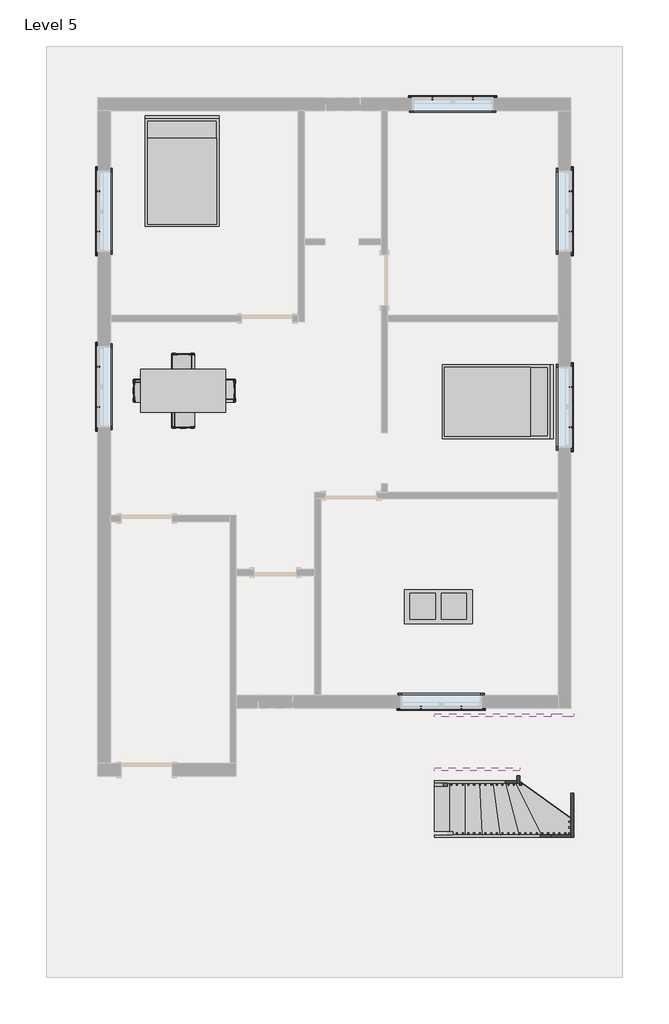
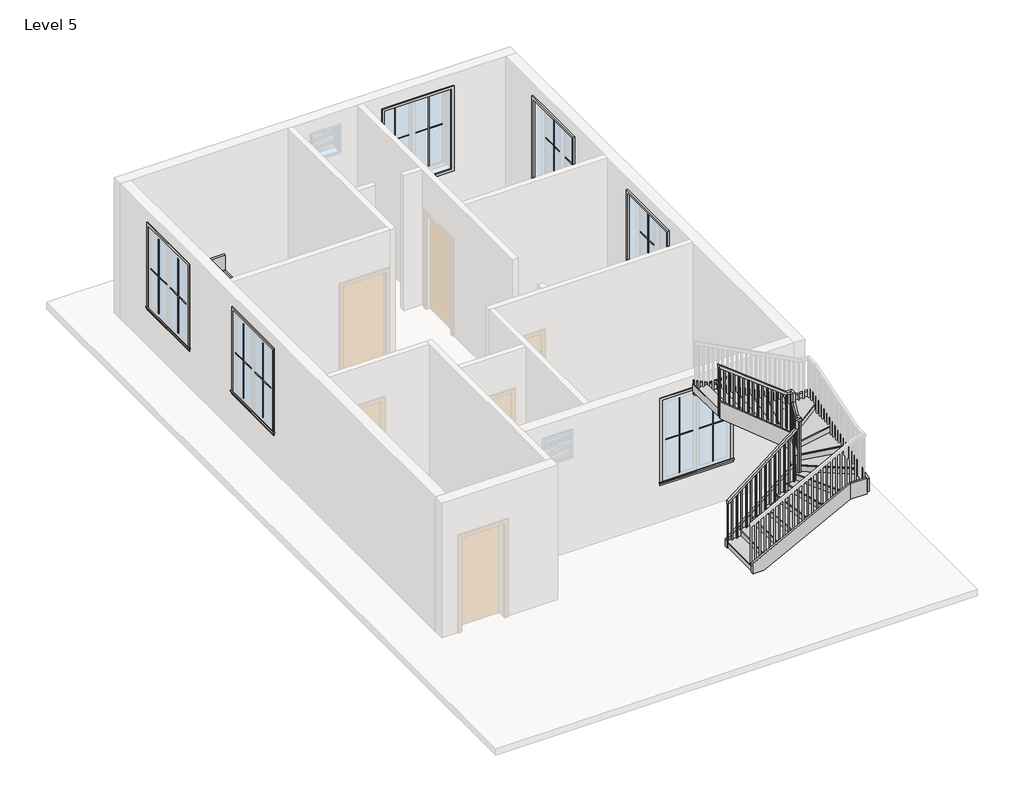
# One storey, part 3 of 3: 25 proxies, 8 members, 3 furniture elements, 1 railing, 1 stair flight.
"""IFC4 building model written with IfcOpenShell, lengths in millimetres."""

from ifc_helpers import new_model, si_unit, frame, origin, place, context, project, spatial, polyline, outline, extrude, faceted_brep, transform, mapped, element, save
from components import muntin_pattern_2x2_muntin_pattern_2x2_bff912c5, muntin_pattern_2x2_muntin_pattern_2x2_c2194282, trim_window_exterior_flat_with_sill_e04b3088, trim_window_interior_flat_picture_frame_2a7685fe, coffee_table_with_brass_mullions_11320_coffee_table_with_5962bef7, bed_17739_bed_17739_15c61121, dining_table_w_chairs_11374_0cdfc61b, stair_flight_5209112f

model = new_model("IFC4")

# Units and contexts
model_context = context("Model", 3, world=origin())
ifc_project = project(units=[si_unit("LENGTHUNIT", "METRE", prefix="MILLI")], contexts=[model_context])

# Site, building, storey
site = spatial("IfcSite", under=ifc_project)
building = spatial("IfcBuilding", under=site)
storey = spatial("IfcBuildingStorey", under=building, Name="Level 5", Elevation=9601.2)

# Proxies
placement = place(None, origin())
muntin_pattern_2x2_muntin_pattern_2x2_shape = muntin_pattern_2x2_muntin_pattern_2x2_bff912c5(model_context)
element("IfcBuildingElementProxy", 1, Name="Muntin Pattern_2x2 : Muntin Pattern_2x2", ObjectType="Muntin Pattern_2x2 : Muntin Pattern_2x2", at=placement, inside=storey, context=model_context, shape_type="MappedRepresentation", body=[
    mapped(muntin_pattern_2x2_muntin_pattern_2x2_shape, transform((2964.3605034, 427.8534591, 10585.45), x_axis=(0.0, -1.0, 0.0), y_axis=(1.0, 0.0, 0.0), z_axis=(0.0, 0.0, 1.0))),
])
element("IfcBuildingElementProxy", 2, Name="Muntin Pattern_2x2 : Muntin Pattern_2x2", ObjectType="Muntin Pattern_2x2 : Muntin Pattern_2x2", at=placement, inside=storey, context=model_context, shape_type="MappedRepresentation", body=[
    mapped(muntin_pattern_2x2_muntin_pattern_2x2_shape, transform((2964.3605034, 3923.5284591, 10585.45), x_axis=(0.0, -1.0, 0.0), y_axis=(1.0, 0.0, 0.0), z_axis=(0.0, 0.0, 1.0))),
])
element("IfcBuildingElementProxy", 3, Name="Muntin Pattern_2x2 : Muntin Pattern_2x2", ObjectType="Muntin Pattern_2x2 : Muntin Pattern_2x2", at=placement, inside=storey, context=model_context, shape_type="MappedRepresentation", body=[
    mapped(muntin_pattern_2x2_muntin_pattern_2x2_shape, transform((498.9730034, 5582.4659591, 10585.45), x_axis=(1.0, 0.0, 0.0), y_axis=(0.0, 1.0, 0.0), z_axis=(0.0, 0.0, 1.0))),
])
element("IfcBuildingElementProxy", 4, Name="Muntin Pattern_2x2 : Muntin Pattern_2x2", ObjectType="Muntin Pattern_2x2 : Muntin Pattern_2x2", at=placement, inside=storey, context=model_context, shape_type="MappedRepresentation", body=[
    mapped(muntin_pattern_2x2_muntin_pattern_2x2_shape, transform((-5474.7894966, 3202.8034591, 10585.45), x_axis=(0.0, 1.0, 0.0), y_axis=(-1.0, 0.0, 0.0), z_axis=(0.0, 0.0, 1.0))),
])
element("IfcBuildingElementProxy", 5, Name="Muntin Pattern_2x2 : Muntin Pattern_2x2", ObjectType="Muntin Pattern_2x2 : Muntin Pattern_2x2", at=placement, inside=storey, context=model_context, shape_type="MappedRepresentation", body=[
    mapped(muntin_pattern_2x2_muntin_pattern_2x2_shape, transform((-5474.7894966, 69.0784591, 10585.45), x_axis=(0.0, 1.0, 0.0), y_axis=(-1.0, 0.0, 0.0), z_axis=(0.0, 0.0, 1.0))),
])
element("IfcBuildingElementProxy", 6, Name="Muntin Pattern_2x2 : Muntin Pattern_2x2", ObjectType="Muntin Pattern_2x2 : Muntin Pattern_2x2", at=placement, inside=storey, context=model_context, shape_type="MappedRepresentation", body=[
    mapped(muntin_pattern_2x2_muntin_pattern_2x2_shape, transform((1013.3230034, -5295.0840409, 10585.45), x_axis=(-1.0, 0.0, 0.0), y_axis=(0.0, -1.0, 0.0), z_axis=(0.0, 0.0, 1.0))),
])
muntin_pattern_2x2_muntin_pattern_2x2_2_shape = muntin_pattern_2x2_muntin_pattern_2x2_c2194282(model_context)
element("IfcBuildingElementProxy", 7, Name="Muntin Pattern_2x2 : Muntin Pattern_2x2", ObjectType="Muntin Pattern_2x2 : Muntin Pattern_2x2", at=placement, inside=storey, context=model_context, shape_type="MappedRepresentation", body=[
    mapped(muntin_pattern_2x2_muntin_pattern_2x2_2_shape, transform((2964.3605034, -292.8715409, 10585.45), x_axis=(0.0, 1.0, 0.0), y_axis=(-1.0, 0.0, 0.0), z_axis=(0.0, 0.0, 1.0))),
])
element("IfcBuildingElementProxy", 8, Name="Muntin Pattern_2x2 : Muntin Pattern_2x2", ObjectType="Muntin Pattern_2x2 : Muntin Pattern_2x2", at=placement, inside=storey, context=model_context, shape_type="MappedRepresentation", body=[
    mapped(muntin_pattern_2x2_muntin_pattern_2x2_2_shape, transform((2964.3605034, 3202.8034591, 10585.45), x_axis=(0.0, 1.0, 0.0), y_axis=(-1.0, 0.0, 0.0), z_axis=(0.0, 0.0, 1.0))),
])
element("IfcBuildingElementProxy", 9, Name="Muntin Pattern_2x2 : Muntin Pattern_2x2", ObjectType="Muntin Pattern_2x2 : Muntin Pattern_2x2", at=placement, inside=storey, context=model_context, shape_type="MappedRepresentation", body=[
    mapped(muntin_pattern_2x2_muntin_pattern_2x2_2_shape, transform((1219.6980034, 5582.4659591, 10585.45), x_axis=(-1.0, 0.0, 0.0), y_axis=(0.0, -1.0, 0.0), z_axis=(0.0, 0.0, 1.0))),
])
element("IfcBuildingElementProxy", 10, Name="Muntin Pattern_2x2 : Muntin Pattern_2x2", ObjectType="Muntin Pattern_2x2 : Muntin Pattern_2x2", at=placement, inside=storey, context=model_context, shape_type="MappedRepresentation", body=[
    mapped(muntin_pattern_2x2_muntin_pattern_2x2_2_shape, transform((-5474.7894966, 3923.5284591, 10585.45), x_axis=(0.0, -1.0, 0.0), y_axis=(1.0, 0.0, 0.0), z_axis=(0.0, 0.0, 1.0))),
])
element("IfcBuildingElementProxy", 11, Name="Muntin Pattern_2x2 : Muntin Pattern_2x2", ObjectType="Muntin Pattern_2x2 : Muntin Pattern_2x2", at=placement, inside=storey, context=model_context, shape_type="MappedRepresentation", body=[
    mapped(muntin_pattern_2x2_muntin_pattern_2x2_2_shape, transform((-5474.7894966, 789.8034591, 10585.45), x_axis=(0.0, -1.0, 0.0), y_axis=(1.0, 0.0, 0.0), z_axis=(0.0, 0.0, 1.0))),
])
element("IfcBuildingElementProxy", 12, Name="Muntin Pattern_2x2 : Muntin Pattern_2x2", ObjectType="Muntin Pattern_2x2 : Muntin Pattern_2x2", at=placement, inside=storey, context=model_context, shape_type="MappedRepresentation", body=[
    mapped(muntin_pattern_2x2_muntin_pattern_2x2_2_shape, transform((292.5980034, -5295.0840409, 10585.45), x_axis=(1.0, 0.0, 0.0), y_axis=(0.0, 1.0, 0.0), z_axis=(0.0, 0.0, 1.0))),
])
trim_window_exterior_flat_with_sill_shape = trim_window_exterior_flat_with_sill_e04b3088(model_context)
element("IfcBuildingElementProxy", 13, Name="Trim-Window-Exterior-Flat : with Sill", ObjectType="Trim-Window-Exterior-Flat : with Sill", at=placement, inside=storey, context=model_context, shape_type="MappedRepresentation", body=[
    mapped(trim_window_exterior_flat_with_sill_shape, transform((2973.8855034, 67.4909591, 12344.4), x_axis=(0.0, 1.0, 0.0), y_axis=(0.0, 0.0, 1.0), z_axis=(1.0, 0.0, 0.0))),
])
element("IfcBuildingElementProxy", 14, Name="Trim-Window-Exterior-Flat : with Sill", ObjectType="Trim-Window-Exterior-Flat : with Sill", at=placement, inside=storey, context=model_context, shape_type="MappedRepresentation", body=[
    mapped(trim_window_exterior_flat_with_sill_shape, transform((2973.8855034, 3563.1659591, 12344.4), x_axis=(0.0, 1.0, 0.0), y_axis=(0.0, 0.0, 1.0), z_axis=(1.0, 0.0, 0.0))),
])
element("IfcBuildingElementProxy", 15, Name="Trim-Window-Exterior-Flat : with Sill", ObjectType="Trim-Window-Exterior-Flat : with Sill", at=placement, inside=storey, context=model_context, shape_type="MappedRepresentation", body=[
    mapped(trim_window_exterior_flat_with_sill_shape, transform((859.3355034, 5591.9909591, 12344.4), x_axis=(-1.0, 0.0, 0.0), y_axis=(0.0, 0.0, 1.0), z_axis=(0.0, 1.0, 0.0))),
])
element("IfcBuildingElementProxy", 16, Name="Trim-Window-Exterior-Flat : with Sill", ObjectType="Trim-Window-Exterior-Flat : with Sill", at=placement, inside=storey, context=model_context, shape_type="MappedRepresentation", body=[
    mapped(trim_window_exterior_flat_with_sill_shape, transform((-5484.3144966, 3563.1659591, 12344.4), x_axis=(0.0, -1.0, 0.0), y_axis=(0.0, 0.0, 1.0), z_axis=(-1.0, 0.0, 0.0))),
])
element("IfcBuildingElementProxy", 17, Name="Trim-Window-Exterior-Flat : with Sill", ObjectType="Trim-Window-Exterior-Flat : with Sill", at=placement, inside=storey, context=model_context, shape_type="MappedRepresentation", body=[
    mapped(trim_window_exterior_flat_with_sill_shape, transform((-5484.3144966, 429.4409591, 12344.4), x_axis=(0.0, -1.0, 0.0), y_axis=(0.0, 0.0, 1.0), z_axis=(-1.0, 0.0, 0.0))),
])
element("IfcBuildingElementProxy", 18, Name="Trim-Window-Exterior-Flat : with Sill", ObjectType="Trim-Window-Exterior-Flat : with Sill", at=placement, inside=storey, context=model_context, shape_type="MappedRepresentation", body=[
    mapped(trim_window_exterior_flat_with_sill_shape, transform((652.9605034, -5304.6090409, 12344.4), x_axis=(1.0, 0.0, 0.0), y_axis=(0.0, 0.0, 1.0), z_axis=(0.0, -1.0, 0.0))),
])
trim_window_interior_flat_picture_frame_shape = trim_window_interior_flat_picture_frame_2a7685fe(model_context)
element("IfcBuildingElementProxy", 19, Name="Trim-Window-Interior-Flat : Picture Frame", ObjectType="Trim-Window-Interior-Flat : Picture Frame", at=placement, inside=storey, context=model_context, shape_type="MappedRepresentation", body=[
    mapped(trim_window_interior_flat_picture_frame_shape, transform((2745.2855034, 67.4909591, 12344.4), x_axis=(0.0, -1.0, 0.0), y_axis=(0.0, 0.0, 1.0), z_axis=(-1.0, 0.0, 0.0))),
])
element("IfcBuildingElementProxy", 20, Name="Trim-Window-Interior-Flat : Picture Frame", ObjectType="Trim-Window-Interior-Flat : Picture Frame", at=placement, inside=storey, context=model_context, shape_type="MappedRepresentation", body=[
    mapped(trim_window_interior_flat_picture_frame_shape, transform((2745.2855034, 3563.1659591, 12344.4), x_axis=(0.0, -1.0, 0.0), y_axis=(0.0, 0.0, 1.0), z_axis=(-1.0, 0.0, 0.0))),
])
element("IfcBuildingElementProxy", 21, Name="Trim-Window-Interior-Flat : Picture Frame", ObjectType="Trim-Window-Interior-Flat : Picture Frame", at=placement, inside=storey, context=model_context, shape_type="MappedRepresentation", body=[
    mapped(trim_window_interior_flat_picture_frame_shape, transform((859.3355034, 5363.3909591, 12344.4), x_axis=(1.0, 0.0, 0.0), y_axis=(0.0, 0.0, 1.0), z_axis=(0.0, -1.0, 0.0))),
])
element("IfcBuildingElementProxy", 22, Name="Trim-Window-Interior-Flat : Picture Frame", ObjectType="Trim-Window-Interior-Flat : Picture Frame", at=placement, inside=storey, context=model_context, shape_type="MappedRepresentation", body=[
    mapped(trim_window_interior_flat_picture_frame_shape, transform((-5255.7144966, 3563.1659591, 12344.4), x_axis=(0.0, 1.0, 0.0), y_axis=(0.0, 0.0, 1.0), z_axis=(1.0, 0.0, 0.0))),
])
element("IfcBuildingElementProxy", 23, Name="Trim-Window-Interior-Flat : Picture Frame", ObjectType="Trim-Window-Interior-Flat : Picture Frame", at=placement, inside=storey, context=model_context, shape_type="MappedRepresentation", body=[
    mapped(trim_window_interior_flat_picture_frame_shape, transform((-5255.7144966, 429.4409591, 12344.4), x_axis=(0.0, 1.0, 0.0), y_axis=(0.0, 0.0, 1.0), z_axis=(1.0, 0.0, 0.0))),
])
element("IfcBuildingElementProxy", 24, Name="Trim-Window-Interior-Flat : Picture Frame", ObjectType="Trim-Window-Interior-Flat : Picture Frame", at=placement, inside=storey, context=model_context, shape_type="MappedRepresentation", body=[
    mapped(trim_window_interior_flat_picture_frame_shape, transform((652.9605034, -5076.0090409, 12344.4), x_axis=(-1.0, 0.0, 0.0), y_axis=(0.0, 0.0, 1.0), z_axis=(0.0, 1.0, 0.0))),
])
coffee_table_with_brass_mullions_11320_coffee_table_with_shape = coffee_table_with_brass_mullions_11320_coffee_table_with_5962bef7(model_context)
element("IfcBuildingElementProxy", 25, Name="coffee_table_with_brass_mullions_11320 : coffee_table_with_brass_mullions_11320", ObjectType="coffee_table_with_brass_mullions_11320 : coffee_table_with_brass_mullions_11320", at=placement, inside=storey, context=model_context, shape_type="MappedRepresentation", body=[
    mapped(coffee_table_with_brass_mullions_11320_coffee_table_with_shape, transform((1240.0943553, -3926.0808329, 9601.2), x_axis=(1.0, 0.0, 0.0), y_axis=(0.0, 1.0, 0.0), z_axis=(0.0, 0.0, 1.0))),
])

# Furniture
bed_17739_bed_17739_shape = bed_17739_bed_17739_15c61121(model_context)
element("IfcFurniture", 26, ObjectType="Bed_17739 : Bed_17739", at=placement, inside=storey, context=model_context, shape_type="MappedRepresentation", body=[
    mapped(bed_17739_bed_17739_shape, transform((-3979.3644966, 4258.4909591, 9601.2), x_axis=(1.0, 0.0, 0.0), y_axis=(0.0, 1.0, 0.0), z_axis=(0.0, 0.0, 1.0))),
])
element("IfcFurniture", 27, ObjectType="Bed_17739 : Bed_17739", at=placement, inside=storey, context=model_context, shape_type="MappedRepresentation", body=[
    mapped(bed_17739_bed_17739_shape, transform((1640.3855034, 162.7409591, 9601.2), x_axis=(0.0, -1.0, 0.0), y_axis=(1.0, 0.0, 0.0), z_axis=(0.0, 0.0, 1.0))),
])
dining_table_w_chairs_11374_shape = dining_table_w_chairs_11374_0cdfc61b(model_context)
element("IfcFurniture", 28, ObjectType="Dining_Table_w_Chairs_11374", at=placement, inside=storey, context=model_context, shape_type="MappedRepresentation", body=[
    mapped(dining_table_w_chairs_11374_shape, transform((-3975.2132663, 265.1952874, 9601.2), x_axis=(1.0, 0.0, 0.0), y_axis=(0.0, 1.0, 0.0), z_axis=(0.0, 0.0, 1.0))),
])

# Members
element("IfcMember", 29, ObjectType="Stringer - 2\" Width", at=placement, inside=storey, context=model_context, shape_type="SweptSolid", body=[
    extrude(outline(polyline([(9777.3764461, 531.7538115), (9601.2, 531.7538115), (9601.2, 798.0154561), (10588.3410923, 2008.6855034), (10981.618648, 2008.6855034), (9777.3764461, 531.7538115)])), frame((0.0, -6650.8090409, 0.0), z_axis=(0.0, 1.0, 0.0), x_axis=(0.0, 0.0, 1.0)), (0.0, 0.0, 1.0), 50.8),
])
element("IfcMember", 30, ObjectType="Stringer - 2\" Width", at=placement, inside=storey, context=model_context, shape_type="SweptSolid", body=[
    extrude(outline(polyline([(-6650.8090409, 10629.7617647), (-6650.8090409, 11174.4682978), (-6444.1719234, 11527.3409689), (-6422.2090409, 11527.3409689), (-6422.2090409, 10961.665107), (-6616.5668235, 10629.7617647), (-6650.8090409, 10629.7617647)])), frame((2008.6855034, 0.0, 0.0), z_axis=(1.0, 0.0, 0.0), x_axis=(0.0, 1.0, 0.0)), (0.0, 0.0, 1.0), 50.8),
])
element("IfcMember", 31, ObjectType="Stringer - 2\" Width", at=placement, inside=storey, context=model_context, shape_type="SweptSolid", body=[
    extrude(outline(polyline([(11134.0634131, 2059.4855034), (11527.3409689, 2059.4855034), (12773.0038432, 531.7538115), (12379.7262875, 531.7538115), (11134.0634131, 2059.4855034)])), frame((0.0, -6422.2090409, 0.0), z_axis=(0.0, 1.0, 0.0), x_axis=(0.0, 0.0, 1.0)), (0.0, 0.0, 1.0), 50.8),
])
element("IfcMember", 32, ObjectType="Stringer - 2\" Width", at=placement, inside=storey, context=model_context, shape_type="SweptSolid", body=[
    extrude(outline(polyline([(9830.839954, 531.7538115), (9601.2, 531.7538115), (9601.2, 751.5161291), (10563.700629, 2619.1710032), (10906.5956453, 2619.1710032), (9830.839954, 531.7538115)])), frame((0.0, -7616.0090409, 0.0), z_axis=(0.0, 1.0, 0.0), x_axis=(0.0, 0.0, 1.0)), (0.0, 0.0, 1.0), 50.8),
])
element("IfcMember", 33, ObjectType="Stringer - 2\" Width", at=placement, inside=storey, context=model_context, shape_type="SweptSolid", body=[
    extrude(outline(polyline([(2619.1710032, -7616.0090409), (2619.1710032, -7565.2090409), (2973.8855034, -7565.2090409), (2973.8855034, -7616.0090409), (2619.1710032, -7616.0090409)])), frame((0.0, 0.0, 10563.700629), z_axis=(0.0, 0.0, 1.0), x_axis=(1.0, 0.0, 0.0)), (0.0, 0.0, 1.0), 342.8950162),
])
element("IfcMember", 34, ObjectType="Stringer - 2\" Width", at=placement, inside=storey, context=model_context, shape_type="SweptSolid", body=[
    extrude(outline(polyline([(-7616.0090409, 10601.7956453), (-7616.0090409, 10890.2952212), (-5493.9891581, 11571.1972697), (-5457.0090409, 11571.1972697), (-5457.0090409, 11240.1682298), (-7446.4865579, 10601.7956453), (-7616.0090409, 10601.7956453)])), frame((2973.8855034, 0.0, 0.0), z_axis=(1.0, 0.0, 0.0), x_axis=(0.0, 1.0, 0.0)), (0.0, 0.0, 1.0), 50.8),
])
element("IfcMember", 35, ObjectType="Stringer - 2\" Width", at=placement, inside=storey, context=model_context, shape_type="SweptSolid", body=[
    extrude(outline(polyline([(3024.6855034, -5406.2090409), (3024.6855034, -5457.0090409), (2619.1710032, -5457.0090409), (2619.1710032, -5406.2090409), (3024.6855034, -5406.2090409)])), frame((0.0, 0.0, 11251.0904473), z_axis=(0.0, 0.0, 1.0), x_axis=(1.0, 0.0, 0.0)), (0.0, 0.0, 1.0), 320.1068224),
])
element("IfcMember", 36, ObjectType="Stringer - 2\" Width", at=placement, inside=storey, context=model_context, shape_type="SweptSolid", body=[
    extrude(outline(polyline([(11251.0904473, 2619.1710032), (11571.1972697, 2619.1710032), (12646.9529609, 531.7538115), (12326.8461385, 531.7538115), (11251.0904473, 2619.1710032)])), frame((0.0, -5457.0090409, 0.0), z_axis=(0.0, 1.0, 0.0), x_axis=(0.0, 0.0, 1.0)), (0.0, 0.0, 1.0), 50.8),
])

# Railing
element("IfcRailing", 37, ObjectType="Handrail - Rectangular", at=placement, inside=storey, context=model_context, shape_type="SolidModel", body=[
    faceted_brep([(531.7538115, -6650.8090409, 10684.9333333), (531.7538115, -6650.8090409, 10620.6000346), (531.7538115, -6701.6090409, 10620.6000346), (531.7538115, -6701.6090409, 10684.9333333), (1983.2855034, -6650.8090409, 11812.8191036), (2034.0855034, -6650.8090409, 11787.9590024), (2034.0855034, -6701.6090409, 11787.9590024), (1983.2855034, -6701.6090409, 11812.8191036), (2059.4855034, -6545.487707, 11965.0281882), (2059.4855034, -6574.6090409, 12015.8281882), (2059.4855034, -6447.6090409, 12232.7051451), (2059.4855034, -6396.8090409, 12218.9256424), (2110.2855034, -6545.487707, 11965.0281882), (2110.2855034, -6396.8090409, 12218.9256424), (2110.2855034, -6574.6090409, 12015.8281882), (2110.2855034, -6447.6090409, 12232.7051451), (531.7538115, -6371.4090409, 13563.6), (531.7538115, -6320.6090409, 13563.6), (531.7538115, -6320.6090409, 13499.2667013), (531.7538115, -6371.4090409, 13499.2667013), (1965.8688354, -6371.4090409, 12384.9142297), (1983.2855034, -6371.4090409, 12435.7142297), (1965.8688354, -6320.6090409, 12384.9142297), (1983.2855034, -6320.6090409, 12435.7142297), (1983.2855034, -6650.8090409, 12015.8281882), (2034.0855034, -6650.8090409, 11965.0281882), (2034.0855034, -6701.6090409, 11965.0281882), (1983.2855034, -6701.6090409, 12015.8281882), (2059.4855034, -6650.8090409, 12015.8281882), (2059.4855034, -6650.8090409, 11965.0281882), (2110.2855034, -6701.6090409, 11965.0281882), (2110.2855034, -6701.6090409, 12015.8281882), (2059.4855034, -6447.6090409, 12435.7142297), (2059.4855034, -6396.8090409, 12384.9142297), (2110.2855034, -6396.8090409, 12384.9142297), (2110.2855034, -6447.6090409, 12435.7142297), (2059.4855034, -6371.4090409, 12435.7142297), (2059.4855034, -6371.4090409, 12384.9142297), (2110.2855034, -6320.6090409, 12384.9142297), (2110.2855034, -6320.6090409, 12435.7142297)], [[[0, 1, 2, 3]], [[1, 0, 4, 5]], [[2, 1, 5, 6]], [[3, 2, 6, 7]], [[0, 3, 7, 4]], [[8, 9, 10, 11]], [[12, 8, 11, 13]], [[14, 12, 13, 15]], [[9, 14, 15, 10]], [[16, 17, 18, 19]], [[20, 21, 16, 19]], [[22, 20, 19, 18]], [[23, 22, 18, 17]], [[21, 23, 17, 16]], [[5, 4, 24, 25]], [[6, 5, 25, 26]], [[7, 6, 26, 27]], [[4, 7, 27, 24]], [[25, 24, 28, 29]], [[26, 25, 29, 30]], [[27, 26, 30, 31]], [[24, 27, 31, 28]], [[29, 28, 9, 8]], [[30, 29, 8, 12]], [[31, 30, 12, 14]], [[28, 31, 14, 9]], [[11, 10, 32, 33]], [[13, 11, 33, 34]], [[15, 13, 34, 35]], [[10, 15, 35, 32]], [[33, 32, 36, 37]], [[34, 33, 37, 38]], [[35, 34, 38, 39]], [[32, 35, 39, 36]], [[37, 36, 21, 20]], [[38, 37, 20, 22]], [[39, 38, 22, 23]], [[36, 39, 23, 21]]]),
    extrude(outline(polyline([(13484.0316852, 551.3605034), (12479.8666667, 551.3605034), (12479.8666667, 570.4105034), (13469.2292361, 570.4105034), (13484.0316852, 551.3605034)])), frame((0.0, -6355.5340409, 0.0), z_axis=(0.0, 1.0, 0.0), x_axis=(0.0, 0.0, 1.0)), (0.0, 0.0, 1.0), 19.05),
    extrude(outline(polyline([(13405.0852902, 652.9605034), (12479.8666667, 652.9605034), (12479.8666667, 672.0105034), (13390.2828411, 672.0105034), (13405.0852902, 652.9605034)])), frame((0.0, -6355.5340409, 0.0), z_axis=(0.0, 1.0, 0.0), x_axis=(0.0, 0.0, 1.0)), (0.0, 0.0, 1.0), 19.05),
    extrude(outline(polyline([(13326.1388952, 754.5605034), (12479.8666667, 754.5605034), (12479.8666667, 773.6105034), (13311.3364462, 773.6105034), (13326.1388952, 754.5605034)])), frame((0.0, -6355.5340409, 0.0), z_axis=(0.0, 1.0, 0.0), x_axis=(0.0, 0.0, 1.0)), (0.0, 0.0, 1.0), 19.05),
    extrude(outline(polyline([(13247.1925003, 856.1605034), (12310.5333333, 856.1605034), (12310.5333333, 875.2105034), (13232.3900512, 875.2105034), (13247.1925003, 856.1605034)])), frame((0.0, -6355.5340409, 0.0), z_axis=(0.0, 1.0, 0.0), x_axis=(0.0, 0.0, 1.0)), (0.0, 0.0, 1.0), 19.05),
    extrude(outline(polyline([(13168.2461053, 957.7605034), (12310.5333333, 957.7605034), (12310.5333333, 976.8105034), (13153.4436562, 976.8105034), (13168.2461053, 957.7605034)])), frame((0.0, -6355.5340409, 0.0), z_axis=(0.0, 1.0, 0.0), x_axis=(0.0, 0.0, 1.0)), (0.0, 0.0, 1.0), 19.05),
    extrude(outline(polyline([(13089.2997103, 1059.3605034), (12310.5333333, 1059.3605034), (12310.5333333, 1078.4105034), (13074.4972613, 1078.4105034), (13089.2997103, 1059.3605034)])), frame((0.0, -6355.5340409, 0.0), z_axis=(0.0, 1.0, 0.0), x_axis=(0.0, 0.0, 1.0)), (0.0, 0.0, 1.0), 19.05),
    extrude(outline(polyline([(13010.3533154, 1160.9605034), (12141.2, 1160.9605034), (12141.2, 1180.0105034), (12995.5508663, 1180.0105034), (13010.3533154, 1160.9605034)])), frame((0.0, -6355.5340409, 0.0), z_axis=(0.0, 1.0, 0.0), x_axis=(0.0, 0.0, 1.0)), (0.0, 0.0, 1.0), 19.05),
    extrude(outline(polyline([(12931.4069204, 1262.5605034), (12141.2, 1262.5605034), (12141.2, 1281.6105034), (12916.6044713, 1281.6105034), (12931.4069204, 1262.5605034)])), frame((0.0, -6355.5340409, 0.0), z_axis=(0.0, 1.0, 0.0), x_axis=(0.0, 0.0, 1.0)), (0.0, 0.0, 1.0), 19.05),
    extrude(outline(polyline([(12852.4605254, 1364.1605034), (11971.8666667, 1364.1605034), (11971.8666667, 1383.2105034), (12837.6580764, 1383.2105034), (12852.4605254, 1364.1605034)])), frame((0.0, -6355.5340409, 0.0), z_axis=(0.0, 1.0, 0.0), x_axis=(0.0, 0.0, 1.0)), (0.0, 0.0, 1.0), 19.05),
    extrude(outline(polyline([(12773.5141304, 1465.7605034), (11971.8666667, 1465.7605034), (11971.8666667, 1484.8105034), (12758.7116814, 1484.8105034), (12773.5141304, 1465.7605034)])), frame((0.0, -6355.5340409, 0.0), z_axis=(0.0, 1.0, 0.0), x_axis=(0.0, 0.0, 1.0)), (0.0, 0.0, 1.0), 19.05),
    extrude(outline(polyline([(12694.5677355, 1567.3605034), (11971.8666667, 1567.3605034), (11971.8666667, 1586.4105034), (12679.7652864, 1586.4105034), (12694.5677355, 1567.3605034)])), frame((0.0, -6355.5340409, 0.0), z_axis=(0.0, 1.0, 0.0), x_axis=(0.0, 0.0, 1.0)), (0.0, 0.0, 1.0), 19.05),
    extrude(outline(polyline([(12615.6213405, 1668.9605034), (11802.5333333, 1668.9605034), (11802.5333333, 1688.0105034), (12600.8188914, 1688.0105034), (12615.6213405, 1668.9605034)])), frame((0.0, -6355.5340409, 0.0), z_axis=(0.0, 1.0, 0.0), x_axis=(0.0, 0.0, 1.0)), (0.0, 0.0, 1.0), 19.05),
    extrude(outline(polyline([(12536.6749455, 1770.5605034), (11802.5333333, 1770.5605034), (11802.5333333, 1789.6105034), (12521.8724965, 1789.6105034), (12536.6749455, 1770.5605034)])), frame((0.0, -6355.5340409, 0.0), z_axis=(0.0, 1.0, 0.0), x_axis=(0.0, 0.0, 1.0)), (0.0, 0.0, 1.0), 19.05),
    extrude(outline(polyline([(12457.7285506, 1872.1605034), (11633.2, 1872.1605034), (11633.2, 1891.2105034), (12442.9261015, 1891.2105034), (12457.7285506, 1872.1605034)])), frame((0.0, -6355.5340409, 0.0), z_axis=(0.0, 1.0, 0.0), x_axis=(0.0, 0.0, 1.0)), (0.0, 0.0, 1.0), 19.05),
    extrude(outline(polyline([(12378.7821556, 1973.7605034), (11633.2, 1973.7605034), (11633.2, 1992.8105034), (12363.9797065, 1992.8105034), (12378.7821556, 1973.7605034)])), frame((0.0, -6355.5340409, 0.0), z_axis=(0.0, 1.0, 0.0), x_axis=(0.0, 0.0, 1.0)), (0.0, 0.0, 1.0), 19.05),
    extrude(outline(polyline([(2075.3605034, -6380.9340409), (2075.3605034, -6361.8840409), (2094.4105034, -6361.8840409), (2094.4105034, -6380.9340409), (2075.3605034, -6380.9340409)])), frame((0.0, 0.0, 11294.5333333), z_axis=(0.0, 0.0, 1.0), x_axis=(1.0, 0.0, 0.0)), (0.0, 0.0, 1.0), 1090.3808964),
    extrude(outline(polyline([(-6463.4840409, 12105.06524), (-6463.4840409, 11125.2), (-6482.5340409, 11125.2), (-6482.5340409, 12072.5336964), (-6463.4840409, 12105.06524)])), frame((2075.3605034, 0.0, 0.0), z_axis=(1.0, 0.0, 0.0), x_axis=(0.0, 1.0, 0.0)), (0.0, 0.0, 1.0), 19.05),
    extrude(outline(polyline([(-6565.0840409, 11931.5636744), (-6565.0840409, 10955.8666667), (-6584.1340409, 10955.8666667), (-6584.1340409, 11899.0321309), (-6565.0840409, 11931.5636744)])), frame((2075.3605034, 0.0, 0.0), z_axis=(1.0, 0.0, 0.0), x_axis=(0.0, 1.0, 0.0)), (0.0, 0.0, 1.0), 19.05),
    extrude(outline(polyline([(2046.2288115, -6666.6840409), (2065.2788115, -6666.6840409), (2065.2788115, -6685.7340409), (2046.2288115, -6685.7340409), (2046.2288115, -6666.6840409)])), frame((0.0, 0.0, 10786.5333333), z_axis=(0.0, 0.0, 1.0), x_axis=(1.0, 0.0, 0.0)), (0.0, 0.0, 1.0), 1178.4948549),
    extrude(outline(polyline([(11718.4483397, 1944.6288115), (10617.2, 1944.6288115), (10617.2, 1963.6788115), (11733.2507888, 1963.6788115), (11718.4483397, 1944.6288115)])), frame((0.0, -6685.7340409, 0.0), z_axis=(0.0, 1.0, 0.0), x_axis=(0.0, 0.0, 1.0)), (0.0, 0.0, 1.0), 19.05),
    extrude(outline(polyline([(11639.5019447, 1843.0288115), (10617.2, 1843.0288115), (10617.2, 1862.0788115), (11654.3043938, 1862.0788115), (11639.5019447, 1843.0288115)])), frame((0.0, -6685.7340409, 0.0), z_axis=(0.0, 1.0, 0.0), x_axis=(0.0, 0.0, 1.0)), (0.0, 0.0, 1.0), 19.05),
    extrude(outline(polyline([(11560.5555498, 1741.4288115), (10447.8666667, 1741.4288115), (10447.8666667, 1760.4788115), (11575.3579988, 1760.4788115), (11560.5555498, 1741.4288115)])), frame((0.0, -6685.7340409, 0.0), z_axis=(0.0, 1.0, 0.0), x_axis=(0.0, 0.0, 1.0)), (0.0, 0.0, 1.0), 19.05),
    extrude(outline(polyline([(11481.6091548, 1639.8288115), (10447.8666667, 1639.8288115), (10447.8666667, 1658.8788115), (11496.4116039, 1658.8788115), (11481.6091548, 1639.8288115)])), frame((0.0, -6685.7340409, 0.0), z_axis=(0.0, 1.0, 0.0), x_axis=(0.0, 0.0, 1.0)), (0.0, 0.0, 1.0), 19.05),
    extrude(outline(polyline([(11402.6627598, 1538.2288115), (10278.5333333, 1538.2288115), (10278.5333333, 1557.2788115), (11417.4652089, 1557.2788115), (11402.6627598, 1538.2288115)])), frame((0.0, -6685.7340409, 0.0), z_axis=(0.0, 1.0, 0.0), x_axis=(0.0, 0.0, 1.0)), (0.0, 0.0, 1.0), 19.05),
    extrude(outline(polyline([(11323.7163649, 1436.6288115), (10278.5333333, 1436.6288115), (10278.5333333, 1455.6788115), (11338.5188139, 1455.6788115), (11323.7163649, 1436.6288115)])), frame((0.0, -6685.7340409, 0.0), z_axis=(0.0, 1.0, 0.0), x_axis=(0.0, 0.0, 1.0)), (0.0, 0.0, 1.0), 19.05),
    extrude(outline(polyline([(11244.7699699, 1335.0288115), (10109.2, 1335.0288115), (10109.2, 1354.0788115), (11259.5724189, 1354.0788115), (11244.7699699, 1335.0288115)])), frame((0.0, -6685.7340409, 0.0), z_axis=(0.0, 1.0, 0.0), x_axis=(0.0, 0.0, 1.0)), (0.0, 0.0, 1.0), 19.05),
    extrude(outline(polyline([(11165.8235749, 1233.4288115), (10109.2, 1233.4288115), (10109.2, 1252.4788115), (11180.626024, 1252.4788115), (11165.8235749, 1233.4288115)])), frame((0.0, -6685.7340409, 0.0), z_axis=(0.0, 1.0, 0.0), x_axis=(0.0, 0.0, 1.0)), (0.0, 0.0, 1.0), 19.05),
    extrude(outline(polyline([(11086.8771799, 1131.8288115), (10109.2, 1131.8288115), (10109.2, 1150.8788115), (11101.679629, 1150.8788115), (11086.8771799, 1131.8288115)])), frame((0.0, -6685.7340409, 0.0), z_axis=(0.0, 1.0, 0.0), x_axis=(0.0, 0.0, 1.0)), (0.0, 0.0, 1.0), 19.05),
    extrude(outline(polyline([(11007.930785, 1030.2288115), (9939.8666667, 1030.2288115), (9939.8666667, 1049.2788115), (11022.733234, 1049.2788115), (11007.930785, 1030.2288115)])), frame((0.0, -6685.7340409, 0.0), z_axis=(0.0, 1.0, 0.0), x_axis=(0.0, 0.0, 1.0)), (0.0, 0.0, 1.0), 19.05),
    extrude(outline(polyline([(10928.98439, 928.6288115), (9939.8666667, 928.6288115), (9939.8666667, 947.6788115), (10943.7868391, 947.6788115), (10928.98439, 928.6288115)])), frame((0.0, -6685.7340409, 0.0), z_axis=(0.0, 1.0, 0.0), x_axis=(0.0, 0.0, 1.0)), (0.0, 0.0, 1.0), 19.05),
    extrude(outline(polyline([(10850.037995, 827.0288115), (9939.8666667, 827.0288115), (9939.8666667, 846.0788115), (10864.8404441, 846.0788115), (10850.037995, 827.0288115)])), frame((0.0, -6685.7340409, 0.0), z_axis=(0.0, 1.0, 0.0), x_axis=(0.0, 0.0, 1.0)), (0.0, 0.0, 1.0), 19.05),
    extrude(outline(polyline([(10771.0916001, 725.4288115), (9770.5333333, 725.4288115), (9770.5333333, 744.4788115), (10785.8940491, 744.4788115), (10771.0916001, 725.4288115)])), frame((0.0, -6685.7340409, 0.0), z_axis=(0.0, 1.0, 0.0), x_axis=(0.0, 0.0, 1.0)), (0.0, 0.0, 1.0), 19.05),
    extrude(outline(polyline([(10692.1452051, 623.8288115), (9770.5333333, 623.8288115), (9770.5333333, 642.8788115), (10706.9476541, 642.8788115), (10692.1452051, 623.8288115)])), frame((0.0, -6685.7340409, 0.0), z_axis=(0.0, 1.0, 0.0), x_axis=(0.0, 0.0, 1.0)), (0.0, 0.0, 1.0), 19.05),
    extrude(outline(polyline([(2075.3605034, -6355.5340409), (2075.3605034, -6336.4840409), (2094.4105034, -6336.4840409), (2094.4105034, -6355.5340409), (2075.3605034, -6355.5340409)])), frame((0.0, 0.0, 11463.8666667), z_axis=(0.0, 0.0, 1.0), x_axis=(1.0, 0.0, 0.0)), (0.0, 0.0, 1.0), 921.0475631),
    extrude(outline(polyline([(2075.3605034, -6666.6840409), (2094.4105034, -6666.6840409), (2094.4105034, -6685.7340409), (2075.3605034, -6685.7340409), (2075.3605034, -6666.6840409)])), frame((0.0, 0.0, 10786.5333333), z_axis=(0.0, 0.0, 1.0), x_axis=(1.0, 0.0, 0.0)), (0.0, 0.0, 1.0), 1178.4948549),
    extrude(outline(polyline([(13499.2667013, 531.7538115), (12479.8666667, 531.7538115), (12479.8666667, 550.8038115), (13484.4642523, 550.8038115), (13499.2667013, 531.7538115)])), frame((0.0, -6355.5340409, 0.0), z_axis=(0.0, 1.0, 0.0), x_axis=(0.0, 0.0, 1.0)), (0.0, 0.0, 1.0), 19.05),
    extrude(outline(polyline([(10620.6000346, 531.7538115), (9770.5333333, 531.7538115), (9770.5333333, 550.8038115), (10635.4024837, 550.8038115), (10620.6000346, 531.7538115)])), frame((0.0, -6685.7340409, 0.0), z_axis=(0.0, 1.0, 0.0), x_axis=(0.0, 0.0, 1.0)), (0.0, 0.0, 1.0), 19.05),
])

# Stair flight
stair_flight_shape = stair_flight_5209112f(model_context)
element("IfcStairFlight", 38, ObjectType="2\" Tread 1\" Nosing 1/4\" Riser", at=placement, inside=storey, context=model_context, shape_type="MappedRepresentation", body=[
    mapped(stair_flight_shape, transform((0.0, 0.0, 0.0), x_axis=(1.0, 0.0, 0.0), y_axis=(0.0, 1.0, 0.0), z_axis=(0.0, 0.0, 1.0))),
])

save(model, "model.ifc")

# Revit data of these elements
# Type "Muntin Pattern_2x2 : Muntin Pattern_2x2"
#   Width [instance default] = 4' - 0"
#   Thickness = 0' - 0 1/2"
#   Height [instance default] = 4' - 0"
#   Distance = 0' - 0 3/4"
#   Interior Material [instance default] = none
#   Exterior Material [instance default] = none
#   Default Elevation = 0
# Type "Trim-Window-Exterior-Flat : with Sill"
#   Trim Width = 0' - 2 1/4"
#   Trim Thickness_Picture Frame = 0' - 1 1/4"
#   Trim Thickness_with Sill = 0' - 0 3/4"
#   Sill Thickness = 0' - 1 1/4"
#   Opening Width [instance default] = 2' - 0"
#   Opening Height [instance default] = 3' - 0"
#   Default Elevation = 4' - 0"
#   Sill = yes
#   Picture Frame = no
#   Trim Material [instance default] = none
# Type "Trim-Window-Interior-Flat : Picture Frame"
#   Trim Thickness_Picture Frame = 0' - 1 1/4"
#   Trim Width = 0' - 2 1/4"
#   Trim Thickness_with Sill = 0' - 0 3/4"
#   Sill Thickness = 0' - 1 1/4"
#   Opening Width [instance default] = 2' - 0"
#   Opening Height [instance default] = 3' - 0"
#   Default Elevation = 4' - 0"
#   Sill = no
#   Picture Frame = yes
#   Trim Material [instance default] = none
# Type "coffee_table_with_brass_mullions_11320 : coffee_table_with_brass_mullions_11320"
#   Default Elevation = 0
# Type "Bed_17739 : Bed_17739"
#   Default Elevation = 0
# Type "Dining_Table_w_Chairs_11374"
#   Default Elevation = 0
#   Assembly Code = ""
# Type "Handrail - Rectangular"
#   Assembly Code = "C2010400"
#   built-in parameter 1008612 = 0.0416667 (stored number, unit not read)
#   built-in parameter 1008611 = 0.0416667 (stored number, unit not read)
#   built-in parameter 1008609 = 0.333333 (stored number, unit not read)
#   built-in parameter 1008604 = 0.166667 (stored number, unit not read)
#   built-in parameter 1008603 = 0.166667 (stored number, unit not read)
#   Railing Height = 3' - 0"
#   built-in parameter 1008630 = 2
#   built-in parameter 1008610 = 2
#   built-in parameter 1008618 = Baluster - Square : 3/4"
# Elements 1, 2, 3, 4, 5, 6, 7, 8, 9, 10, 11, 12 (IfcBuildingElementProxy, "Muntin Pattern_2x2 : Muntin Pattern_2x2")
#   Width = 1' - 11 1/8"
#   Height = 5' - 6 1/2"
#   Interior Material = Wood - Stained
#   Exterior Material = Clad - White
#   Phase Created = New Construction
#   Materials on its faces: "Clad - White", "Wood - Stained"
# Elements 13, 14, 15, 16, 17, 18 (IfcBuildingElementProxy, "Trim-Window-Exterior-Flat : with Sill")
#   Opening Width = 4' - 9"
#   Opening Height = 6' - 0"
#   Trim Material = Clad - White
#   Phase Created = New Construction
#   Materials on its faces: "Clad - White"
# Elements 19, 20, 21, 22, 23, 24 (IfcBuildingElementProxy, "Trim-Window-Interior-Flat : Picture Frame")
#   Opening Width = 4' - 9"
#   Opening Height = 6' - 0"
#   Trim Material = Wood - Stained
#   Phase Created = New Construction
#   Materials on its faces: "Wood - Stained"
# Element 25 (IfcBuildingElementProxy, "coffee_table_with_brass_mullions_11320 : coffee_table_with_brass_mullions_11320")
#   Phase Created = New Construction
#   Materials on its faces: "Default Wall", "TABLE", "Glass", "Default"
# Elements 26, 27 (IfcFurniture, "Bed_17739 : Bed_17739")
#   Phase Created = New Construction
#   Materials on its faces: "legs", "sheets", "bed frame", "Blanket"
# Element 28 (IfcFurniture, "Dining_Table_w_Chairs_11374")
#   Phase Created = New Construction
# Elements 29, 30, 31, 32, 33, 34, 35, 36 (IfcMember, "Stringer - 2\" Width")
#   Phase Created = New Construction
# Element 37 (IfcRailing, "Handrail - Rectangular")
#   Phase Created = New Construction
# Element 38 (IfcStairFlight, "2\" Tread 1\" Nosing 1/4\" Riser")
#   Phase Created = New Construction
# Materials
#   "Clad - White": class "Wood", colour RGB 242 242 238, transparency 0, Cost = 0
#   "Wood - Stained": class "Wood", colour RGB 224 178 126, transparency 0, Cost = 0
#   "Default Wall": colour RGB 128 128 128, transparency 0, Cost = 0
#   "TABLE": class "Generic", colour RGB 120 120 120, transparency 0, Cost = 0
#   "Glass": class "Glass", colour RGB 0 128 192, transparency 0.75, Description = "Soda Lime Glass", Cost = 0
#   "Default": colour RGB 127 127 127, transparency 0, Cost = 0
#   "legs": colour RGB 90 73 37, transparency 0, Cost = 0
#   "sheets": colour RGB 200 195 176, transparency 0, Cost = 0
#   "bed frame": colour RGB 90 73 37, transparency 0, Cost = 0
#   "Blanket": class "System", colour RGB 59 0 1, transparency 0, Cost = 0
